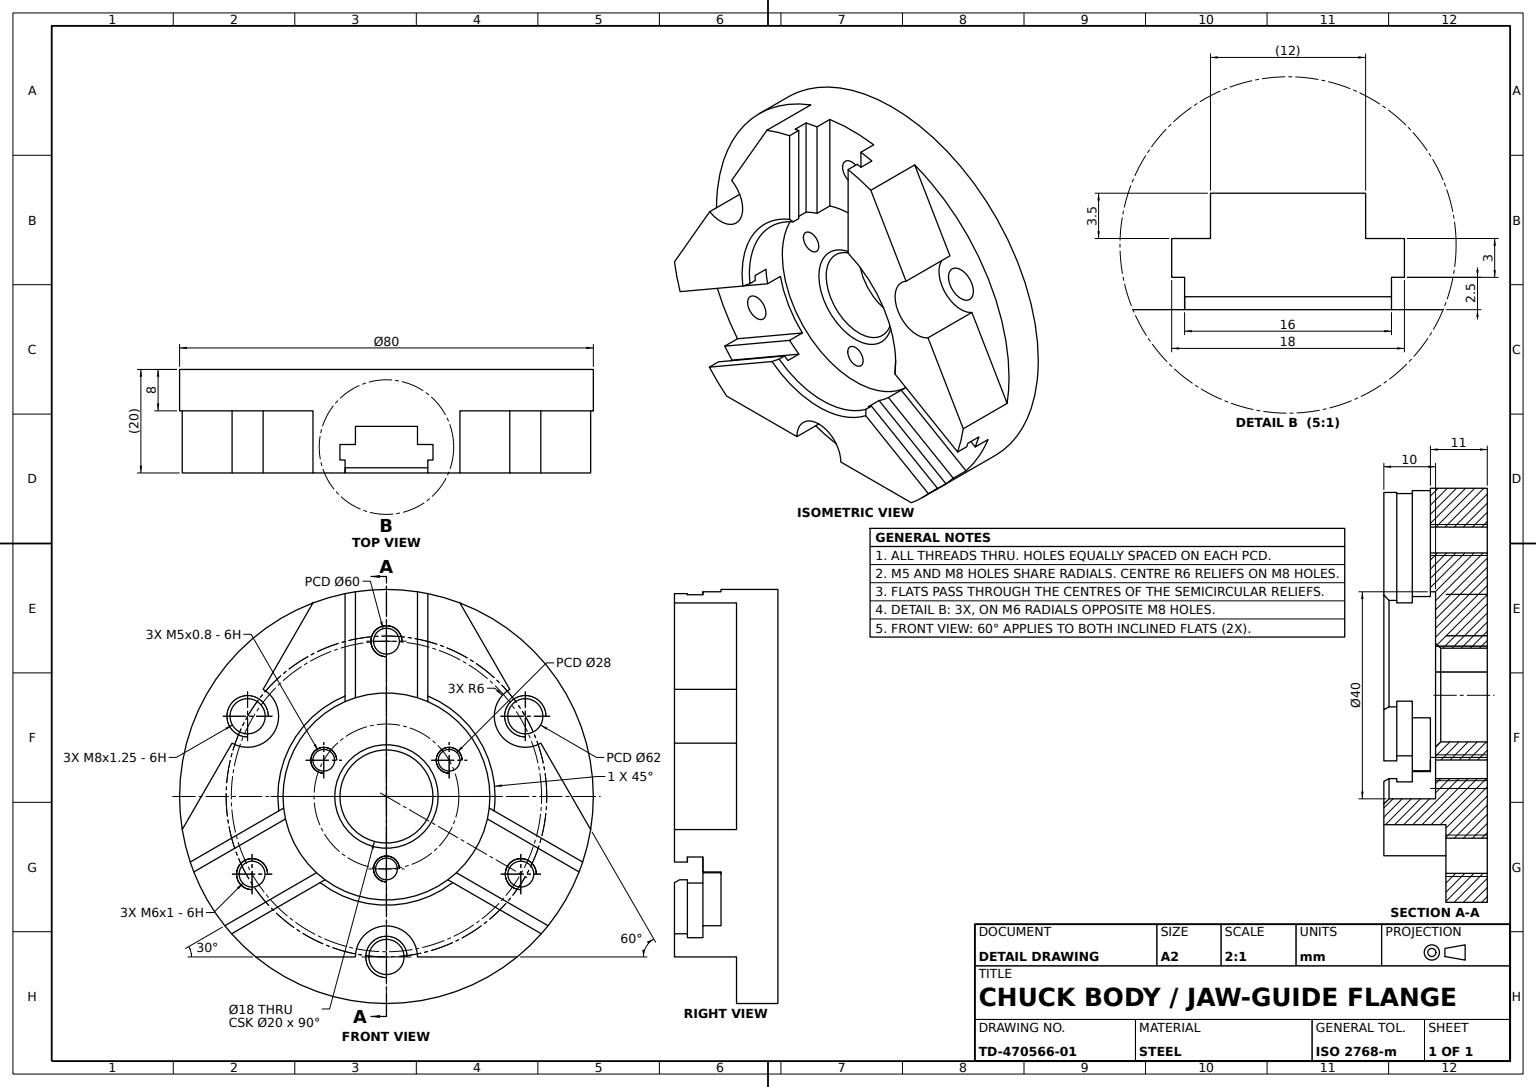
from build123d import *

# Parameters (mm, degrees)
FLANGE_AND_SPOKE_PROFILE_SKETCH_R = 40
FLANGE_DISC_80_DEPTH              = 8
SPOKES_START                      = 8
SPOKES_3X_DEPTH                   = 12
CENTRE_RECESS_SKETCH_40_R         = 20
CENTRE_RECESS_40_DEPTH            = 10
LOCKING_START                     = 17.5
LOCKING_SLOT_STEP_2_5MM_DEPTH     = 2.5
LOCKING_START_2                   = 14.5
LOCKING_SLOT_STEP_3MM_DEPTH       = 3
LOCKING_START_3                   = 11
LOCKING_SLOT_STEP_3_5MM_DEPTH     = 3.5
LOCKING_SLOT_PATTERN_3X_COUNT     = 3
BORE_SKETCH_18_R                  = 9
BORE_18_DEPTH                     = 17
TAPPED_HOLES_3XM5_PCD28_D         = 4.2
TAPPED_HOLES_3XM6_PCD60_D         = 5
TAPPED_HOLES_3XM8_PCD62_D         = 6.8
EDGE_CHAMFER_1X45_SIZE            = 1


with BuildPart() as part:
    # Flange and Spoke Profile Sketch → Flange Disc _80 (new body)
    with BuildSketch(Plane.XY):
        Circle(FLANGE_AND_SPOKE_PROFILE_SKETCH_R)
    extrude(amount=FLANGE_DISC_80_DEPTH)

    # Sketch1_3 → Spokes 3x (add)
    with BuildSketch(Plane.XY.offset(SPOKES_START)):
        with BuildLine():
            Line((-29.846787517, 10.303847577), (-39.486012177, -6.391779279))
            ThreePointArc((-39.486012177, -6.391779279), (-34.641016151, -20), (-25.27844932, -31))
            Line((-25.27844932, -31), (-6, -31))
            ThreePointArc((-6, -31), (0, -25), (6, -31))
            Line((6, -31), (25.27844932, -31))
            ThreePointArc((25.27844932, -31), (34.641016151, -20), (39.486012177, -6.391779279))
            Line((39.486012177, -6.391779279), (29.846787517, 10.303847577))
            ThreePointArc((29.846787517, 10.303847577), (21.650635095, 12.5), (23.846787517, 20.696152423))
            Line((23.846787517, 20.696152423), (14.207562858, 37.391779279))
            ThreePointArc((14.207562858, 37.391779279), (0, 40), (-14.207562858, 37.391779279))
            Line((-14.207562858, 37.391779279), (-23.846787517, 20.696152423))
            ThreePointArc((-23.846787517, 20.696152423), (-21.650635095, 12.5), (-29.846787517, 10.303847577))
        make_face()
    extrude(amount=SPOKES_3X_DEPTH)

    # Centre Recess Sketch _40 → Centre Recess _40 (cut)
    with BuildSketch(Plane.XY.offset(20)):
        Circle(CENTRE_RECESS_SKETCH_40_R)
    extrude(amount=-CENTRE_RECESS_40_DEPTH, mode=Mode.SUBTRACT)

    # Locking Slot Sketch → Locking Slot Step 2.5mm (cut)
    with BuildSketch(Plane.XY.offset(LOCKING_START)):
        with BuildLine():
            Line((37.249087579, -14.577567511), (19.522711642, -4.343239591))
            ThreePointArc((19.522711642, -4.343239591), (17.320508076, -10), (13.522711642, -14.735544437))
            Line((13.522711642, -14.735544437), (31.249087579, -24.969872356))
            ThreePointArc((31.249087579, -24.969872356), (34.641016151, -20), (37.249087579, -14.577567511))
        make_face()
        with BuildLine():
            Line((31.249087579, -24.969872356), (13.522711642, -14.735544437))
            ThreePointArc((13.522711642, -14.735544437), (12.716744938, -15.436463267), (11.874507866, -16.09335462))
            Line((11.874507866, -16.09335462), (29.941125497, -26.524121173))
            ThreePointArc((29.941125497, -26.524121173), (30.604974537, -25.755301077), (31.249087579, -24.969872356))
        make_face()
        with BuildLine():
            ThreePointArc((19.874507866, -2.23694816), (19.726741803, -3.294792536), (19.522711642, -4.343239591))
            Line((19.522711642, -4.343239591), (37.249087579, -14.577567511))
            ThreePointArc((37.249087579, -14.577567511), (37.607232284, -13.627034893), (37.941125497, -12.667714712))
            Line((37.941125497, -12.667714712), (19.874507866, -2.23694816))
        make_face()
    locking_slot_step_2_5mm = extrude(amount=LOCKING_SLOT_STEP_2_5MM_DEPTH, mode=Mode.SUBTRACT)

    # Sketch5_3 → Locking Slot Step 3mm (cut)
    with BuildSketch(Plane.XY.offset(LOCKING_START_2)):
        with BuildLine():
            Line((37.249087579, -14.577567511), (19.522711642, -4.343239591))
            ThreePointArc((19.522711642, -4.343239591), (17.320508076, -10), (13.522711642, -14.735544437))
            Line((13.522711642, -14.735544437), (31.249087579, -24.969872356))
            ThreePointArc((31.249087579, -24.969872356), (34.641016151, -20), (37.249087579, -14.577567511))
        make_face()
        with BuildLine():
            ThreePointArc((19.874507866, -2.23694816), (19.726741803, -3.294792536), (19.522711642, -4.343239591))
            Line((19.522711642, -4.343239591), (37.249087579, -14.577567511))
            ThreePointArc((37.249087579, -14.577567511), (37.607232284, -13.627034893), (37.941125497, -12.667714712))
            Line((37.941125497, -12.667714712), (19.874507866, -2.23694816))
        make_face()
        with BuildLine():
            ThreePointArc((19.967708298, -1.136056916), (19.928711389, -1.687146227), (19.874507866, -2.23694816))
            Line((19.874507866, -2.23694816), (37.941125497, -12.667714712))
            ThreePointArc((37.941125497, -12.667714712), (38.100069067, -12.181327395), (38.252777663, -11.692946636))
            Line((38.252777663, -11.692946636), (19.967708298, -1.136056916))
        make_face()
        with BuildLine():
            Line((31.249087579, -24.969872356), (13.522711642, -14.735544437))
            ThreePointArc((13.522711642, -14.735544437), (12.716744938, -15.436463267), (11.874507866, -16.09335462))
            Line((11.874507866, -16.09335462), (29.941125497, -26.524121173))
            ThreePointArc((29.941125497, -26.524121173), (30.604974537, -25.755301077), (31.249087579, -24.969872356))
        make_face()
        with BuildLine():
            Line((29.941125497, -26.524121173), (11.874507866, -16.09335462))
            ThreePointArc((11.874507866, -16.09335462), (11.425467186, -16.415197214), (10.967708298, -16.724514184))
            Line((10.967708298, -16.724514184), (29.252777663, -27.281403904))
            ThreePointArc((29.252777663, -27.281403904), (29.599373509, -26.904964001), (29.941125497, -26.524121173))
        make_face()
    locking_slot_step_3mm = extrude(amount=LOCKING_SLOT_STEP_3MM_DEPTH, mode=Mode.SUBTRACT)

    # Sketch5_4 → Locking Slot Step 3.5mm (cut)
    with BuildSketch(Plane.XY.offset(LOCKING_START_3)):
        with BuildLine():
            Line((37.249087579, -14.577567511), (19.522711642, -4.343239591))
            ThreePointArc((19.522711642, -4.343239591), (17.320508076, -10), (13.522711642, -14.735544437))
            Line((13.522711642, -14.735544437), (31.249087579, -24.969872356))
            ThreePointArc((31.249087579, -24.969872356), (34.641016151, -20), (37.249087579, -14.577567511))
        make_face()
    locking_slot_step_3_5mm = extrude(amount=LOCKING_SLOT_STEP_3_5MM_DEPTH, mode=Mode.SUBTRACT)

    # Locking Slot Pattern 3x: Locking Slot Step 2.5mm, Locking Slot Step 3mm, Locking Slot Step 3.5mm ×3 about axis
    locking_slot_pattern_3x_axis = Axis((0, 0, 0), (0, 0, 1))
    add([locking_slot_step_2_5mm.rotate(locking_slot_pattern_3x_axis, i * 360 / LOCKING_SLOT_PATTERN_3X_COUNT) for i in range(1, LOCKING_SLOT_PATTERN_3X_COUNT)], mode=Mode.SUBTRACT)
    add([locking_slot_step_3mm.rotate(locking_slot_pattern_3x_axis, i * 360 / LOCKING_SLOT_PATTERN_3X_COUNT) for i in range(1, LOCKING_SLOT_PATTERN_3X_COUNT)], mode=Mode.SUBTRACT)
    add([locking_slot_step_3_5mm.rotate(locking_slot_pattern_3x_axis, i * 360 / LOCKING_SLOT_PATTERN_3X_COUNT) for i in range(1, LOCKING_SLOT_PATTERN_3X_COUNT)], mode=Mode.SUBTRACT)

    # Bore Sketch _18 → Bore _18 (cut)
    with BuildSketch(Plane.XY.offset(10)):
        Circle(BORE_SKETCH_18_R)
    extrude(amount=-BORE_18_DEPTH, mode=Mode.SUBTRACT)

    # Tapped Holes 3xM5 PCD28 (through all)
    with Locations(Plane.XY.offset(10)):
        with Locations((12.124355653, 7), (0, -14), (-12.124355653, 7)):
            Hole(TAPPED_HOLES_3XM5_PCD28_D / 2)

    # Tapped Holes 3xM6 PCD60 (through all)
    with Locations(Plane.XY.offset(11)):
        with Locations((-25.980762114, -15), (0, 30), (25.980762114, -15)):
            Hole(TAPPED_HOLES_3XM6_PCD60_D / 2)

    # Tapped Holes 3xM8 PCD62 (through all)
    with Locations(Plane.XY.offset(8)):
        with Locations((26.846787517, 15.5), (0, -31), (-26.846787517, 15.5)):
            Hole(TAPPED_HOLES_3XM8_PCD62_D / 2)

    # Edge Chamfer 1x45
    edge_chamfer_1x45_edges = [part.edges().sort_by_distance(p)[0] for p in [
        (-17.320508076, 10, 20),
        (0, -20, 20),
        (-9, 0, 10),
        (16.733200531, 10.95445115, 20),
    ]]
    chamfer(edge_chamfer_1x45_edges, length=EDGE_CHAMFER_1X45_SIZE)


solid = part.part
